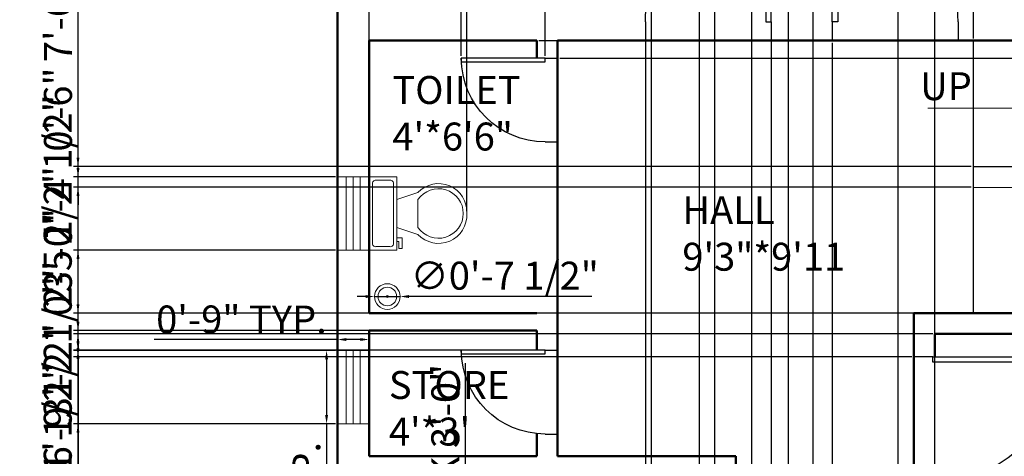
# Model space of a CAD drawing. Units: inches. Extents: x 2528 to 2954, y 1660 to 2209.
# Tile 2 of 4: x 2528 to 2810, y 1832 to 1957. Entities that reach past the tile are written whole.
import ezdxf

# ---------------------------------------------------------------- set-up
doc = ezdxf.new("R2010")
doc.units = ezdxf.units.IN
for name, color, linetype, lineweight in [('A-ANNO-DIMS', 5, 'Continuous', 18), ('A-ANNO-SYMB', 5, 'Continuous', 18), ('A-AREA-IDEN', 5, 'Continuous', 25), ('A-FLOR-FIXT', 6, 'Continuous', 18), ('DOOR', 3, 'Continuous', 25), ('STEPS', 30, 'Continuous', 25), ('TEXT', 5, 'Continuous', 25), ('WALL', 1, 'Continuous', 50), ('WINDOW', 4, 'Continuous', 18)]:
    doc.layers.add(name, color=color, linetype=linetype, lineweight=lineweight)
doc.styles.get("Standard").update_dxf_attribs({"font": 'arial.ttf'})
doc.dimstyles.new('ISO-25', dxfattribs={"dimtxt": 8, "dimasz": 2.5, "dimexe": 1.25, "dimexo": 0.625, "dimtad": 1, "dimlunit": 3, "dimtxsty": 'Standard', "dimcen": 2.5, "dimadec": 0, "dimazin": 0, "dimtfac": 1, "dimtmove": 0, "dimatfit": 3, "dimfxl": 1, "dimarcsym": 0})

# ---------------------------------------------------------------- blocks, each defined once
blk = doc.blocks.new('*U2')
for p, q in [((0, 0), (0, -6)), ((40, 0), (40, -6))]:
    blk.add_line(p, q)
blk.add_lwpolyline([(0, 0), (0, 40), (1.75, 40), (1.75, 0)], close=True)
blk.add_arc((0, 0), 40, 0, 90)
blk = doc.blocks.new('*U4')
for p, q in [((9.5, -6), (9.5, -2)), ((-8, -8.5), (-8, -8)), ((-7, -8), (-7, -9.5)), ((-4, -8), (-6, -14)), ((4, -8), (6, -14)), ((-10, -8.5), (-8, -8.5)), ((-10, -9.5), (-10, -8.5)), ((-7, -9.5), (-10, -9.5)), ((4, -14), (-4, -14))]:
    blk.add_line(p, q)
blk.add_lwpolyline([(10.5, -8), (10.5, 0), (-10.5, 0), (-10.5, -8)], close=True)
for points in [[(-9.5, -2), (-9.5, -6)], [(8.5, -1), (-8.5, -1)], [(-8.5, -7), (8.5, -7)]]:
    blk.add_lwpolyline(points)
for centre, radius, start, end in [((-8.625, -1.875), 0.8839, 81.8699, 188.1301), ((8.625, -1.875), 0.8839, 351.8699, 98.1301), ((-8.625, -6.125), 0.8839, 171.869898, 278.1301), ((8.625, -6.125), 0.8839, 261.8699, 8.1301), ((-0.4772, -19.9188), 8.0953, 133.01722, 273.38), ((0.0374, -19.8731), 7.127, 124.50543, 269.7), ((-0.0373, -19.8731), 7.127, 270.3, 55.4946), ((0.4773, -19.9188), 8.0953, 266.62, 46.9828)]:
    blk.add_arc(centre, radius, start, end)
blk = doc.blocks.new('WIN-21IN')
for p, q in [((9, 21), (0, 21)), ((2.5, 21), (2.5, 0)), ((4.5, 21), (4.5, 0)), ((6.5, 21), (6.5, 0)), ((9, 0), (0, 0))]:
    blk.add_line(p, q)
blk = doc.blocks.new('*D19')
at = {"layer": 'A-ANNO-DIMS', "color": 0, "lineweight": -2, "transparency": 16777216}
for p, q in [((2618.29, 1862.65), (2614.52, 1862.65)), ((2615.77, 1860.15), (2615.77, 1844.15)), ((2618.29, 1841.65), (2614.52, 1841.65)), ((2615.77, 1841.65), (2615.77, 1736.66))]:
    blk.add_line(p, q, dxfattribs=at)
at = {"layer": 'A-ANNO-DIMS', "color": 0, "transparency": 16777216}
for points in [[(2615.35, 1860.15), (2616.18, 1860.15), (2615.77, 1862.65)], [(2615.35, 1844.15), (2616.18, 1844.15), (2615.77, 1841.65)]]:
    blk.add_solid(points, dxfattribs=at)
at = {"layer": 'Defpoints', "color": 0, "transparency": 16777216}
for p in [(2618.92, 1862.65), (2615.77, 1841.65), (2618.92, 1841.65)]:
    blk.add_point(p, dxfattribs=at)
at = {"layer": 'A-ANNO-DIMS', "color": 0, "transparency": 16777216, "insert": (2611, 1787.9), "char_height": 8, "attachment_point": 5, "rotation": 90}
blk.add_mtext('WINDOW 1\'-9" TYP.', dxfattribs=at)
blk = doc.blocks.new('*D20')
at = {"layer": 'A-ANNO-DIMS', "color": 0, "lineweight": -2, "transparency": 16777216}
for p, q in [((2618.92, 1863.27), (2618.92, 1867.05)), ((2627.92, 1863.27), (2627.92, 1867.05)), ((2618.92, 1865.8), (2566.4, 1865.8)), ((2625.42, 1865.8), (2621.42, 1865.8))]:
    blk.add_line(p, q, dxfattribs=at)
at = {"layer": 'A-ANNO-DIMS', "color": 0, "transparency": 16777216}
for points in [[(2621.42, 1866.21), (2621.42, 1865.38), (2618.92, 1865.8)], [(2625.42, 1866.21), (2625.42, 1865.38), (2627.92, 1865.8)]]:
    blk.add_solid(points, dxfattribs=at)
at = {"layer": 'Defpoints', "color": 0, "transparency": 16777216}
for p in [(2618.92, 1865.8), (2618.92, 1862.65), (2627.92, 1862.65)]:
    blk.add_point(p, dxfattribs=at)
at = {"layer": 'A-ANNO-DIMS', "color": 0, "transparency": 16777216, "insert": (2591.41, 1870.5), "char_height": 8, "attachment_point": 5}
blk.add_mtext('0\'-9" TYP.', dxfattribs=at)
blk = doc.blocks.new('*D23')
at = {"layer": 'A-ANNO-DIMS', "color": 0, "lineweight": -2, "transparency": 16777216}
for p, q in [((2655.56, 1804.89), (2655.56, 1859.06)), ((2650.79, 1804.89), (2656.81, 1804.89)), ((2655.56, 1771.39), (2655.56, 1802.39)), ((2650.79, 1768.89), (2656.81, 1768.89))]:
    blk.add_line(p, q, dxfattribs=at)
at = {"layer": 'A-ANNO-DIMS', "color": 0, "transparency": 16777216}
for points in [[(2655.15, 1802.39), (2655.98, 1802.39), (2655.56, 1804.89)], [(2655.15, 1771.39), (2655.98, 1771.39), (2655.56, 1768.89)]]:
    blk.add_solid(points, dxfattribs=at)
at = {"layer": 'Defpoints', "color": 0, "transparency": 16777216}
for p in [(2650.16, 1804.89), (2655.56, 1804.89), (2650.16, 1768.89)]:
    blk.add_point(p, dxfattribs=at)
at = {"layer": 'A-ANNO-DIMS', "color": 0, "transparency": 16777216, "insert": (2650.8, 1833.22), "char_height": 8, "attachment_point": 5, "rotation": 90}
blk.add_mtext('SINK 3\'-0"', dxfattribs=at)
blk = doc.blocks.new('*D28')
at = {"layer": 'A-ANNO-DIMS', "color": 0, "lineweight": -2, "transparency": 16777216}
for p, q in [((2544.62, 1841.65), (2544.62, 1885.3)), ((2618.29, 1841.65), (2543.37, 1841.65)), ((2544.62, 1805.43), (2544.62, 1839.14)), ((2618.29, 1802.93), (2543.37, 1802.93))]:
    blk.add_line(p, q, dxfattribs=at)
at = {"layer": 'A-ANNO-DIMS', "color": 0, "transparency": 16777216}
for points in [[(2544.2, 1839.14), (2545.03, 1839.14), (2544.62, 1841.65)], [(2544.2, 1805.43), (2545.03, 1805.43), (2544.62, 1802.93)]]:
    blk.add_solid(points, dxfattribs=at)
at = {"layer": 'Defpoints', "color": 0, "transparency": 16777216}
for p in [(2544.62, 1841.65), (2618.92, 1841.65), (2618.92, 1802.93)]:
    blk.add_point(p, dxfattribs=at)
at = {"layer": 'A-ANNO-DIMS', "color": 0, "transparency": 16777216, "insert": (2539.85, 1864.72), "char_height": 8, "attachment_point": 5, "rotation": 90}
blk.add_mtext('3\'-2 1/2"', dxfattribs=at)
blk = doc.blocks.new('*D29')
at = {"layer": 'A-ANNO-DIMS', "color": 0, "lineweight": -2, "transparency": 16777216}
for p, q in [((2544.62, 1891.39), (2544.62, 1935.18)), ((2618.29, 1891.39), (2543.37, 1891.39)), ((2544.62, 1865.15), (2544.62, 1888.89)), ((2618.29, 1862.64), (2543.37, 1862.64))]:
    blk.add_line(p, q, dxfattribs=at)
at = {"layer": 'A-ANNO-DIMS', "color": 0, "transparency": 16777216}
for points in [[(2544.2, 1888.89), (2545.03, 1888.89), (2544.62, 1891.39)], [(2544.2, 1865.15), (2545.03, 1865.15), (2544.62, 1862.64)]]:
    blk.add_solid(points, dxfattribs=at)
at = {"layer": 'Defpoints', "color": 0, "transparency": 16777216}
for p in [(2544.62, 1891.39), (2618.92, 1891.39), (2618.92, 1862.64)]:
    blk.add_point(p, dxfattribs=at)
at = {"layer": 'A-ANNO-DIMS', "color": 0, "transparency": 16777216, "insert": (2539.85, 1914.54), "char_height": 8, "attachment_point": 5, "rotation": 90}
blk.add_mtext('2\'-4 1/2"', dxfattribs=at)
blk = doc.blocks.new('*D30')
at = {"layer": 'A-ANNO-DIMS', "color": 0, "lineweight": -2, "transparency": 16777216}
for p, q in [((2618.29, 2002.2), (2543.37, 2002.2)), ((2544.62, 1914.89), (2544.62, 1999.7)), ((2618.29, 1912.39), (2543.37, 1912.39))]:
    blk.add_line(p, q, dxfattribs=at)
at = {"layer": 'A-ANNO-DIMS', "color": 0, "transparency": 16777216}
for points in [[(2544.2, 1999.7), (2545.03, 1999.7), (2544.62, 2002.2)], [(2544.2, 1914.89), (2545.03, 1914.89), (2544.62, 1912.39)]]:
    blk.add_solid(points, dxfattribs=at)
at = {"layer": 'Defpoints', "color": 0, "transparency": 16777216}
for p in [(2544.62, 2002.2), (2618.92, 2002.2), (2618.92, 1912.39)]:
    blk.add_point(p, dxfattribs=at)
at = {"layer": 'A-ANNO-DIMS', "color": 0, "transparency": 16777216, "insert": (2539.91, 1957.29), "char_height": 8, "attachment_point": 5, "rotation": 90}
blk.add_mtext('7\'-6"', dxfattribs=at)
blk = doc.blocks.new('*D34')
at = {"layer": 'A-ANNO-DIMS', "color": 0, "lineweight": -2, "transparency": 16777216}
for p, q in [((2618.92, 1715.01), (2618.92, 2122.94)), ((2726.92, 1703.01), (2726.92, 2122.94)), ((2621.42, 2121.69), (2724.42, 2121.69))]:
    blk.add_line(p, q, dxfattribs=at)
at = {"layer": 'A-ANNO-DIMS', "color": 0, "transparency": 16777216}
for points in [[(2621.42, 2122.11), (2621.42, 2121.27), (2618.92, 2121.69)], [(2724.42, 2122.11), (2724.42, 2121.27), (2726.92, 2121.69)]]:
    blk.add_solid(points, dxfattribs=at)
at = {"layer": 'Defpoints', "color": 0, "transparency": 16777216}
for p in [(2726.92, 2121.69), (2618.92, 1714.39), (2726.92, 1702.39)]:
    blk.add_point(p, dxfattribs=at)
at = {"layer": 'A-ANNO-DIMS', "color": 0, "transparency": 16777216, "insert": (2672.92, 2126.4), "char_height": 8, "attachment_point": 5}
blk.add_mtext('9\'-0"', dxfattribs=at)
blk = doc.blocks.new('*D35')
at = {"layer": 'A-ANNO-DIMS', "color": 0, "lineweight": -2, "transparency": 16777216}
for p, q in [((2726.92, 1691.01), (2726.92, 2122.94)), ((2789.92, 1691.01), (2789.92, 2122.94)), ((2729.42, 2121.69), (2787.42, 2121.69))]:
    blk.add_line(p, q, dxfattribs=at)
at = {"layer": 'A-ANNO-DIMS', "color": 0, "transparency": 16777216}
for points in [[(2729.42, 2122.11), (2729.42, 2121.27), (2726.92, 2121.69)], [(2787.42, 2122.11), (2787.42, 2121.27), (2789.92, 2121.69)]]:
    blk.add_solid(points, dxfattribs=at)
at = {"layer": 'Defpoints', "color": 0, "transparency": 16777216}
for p in [(2789.92, 2121.69), (2726.92, 1690.39), (2789.92, 1690.39)]:
    blk.add_point(p, dxfattribs=at)
at = {"layer": 'A-ANNO-DIMS', "color": 0, "transparency": 16777216, "insert": (2758.42, 2126.4), "char_height": 8, "attachment_point": 5}
blk.add_mtext('5\'-3"', dxfattribs=at)
blk = doc.blocks.new('*D37')
at = {"layer": 'A-ANNO-DIMS', "color": 0, "lineweight": -2, "transparency": 16777216}
for p, q in [((2737.46, 1724.01), (2737.46, 2122.94)), ((2779.37, 1724.01), (2779.37, 2122.94)), ((2739.96, 2121.69), (2776.87, 2121.69))]:
    blk.add_line(p, q, dxfattribs=at)
at = {"layer": 'A-ANNO-DIMS', "color": 0, "transparency": 16777216}
for points in [[(2739.96, 2122.11), (2739.96, 2121.27), (2737.46, 2121.69)], [(2776.87, 2122.11), (2776.87, 2121.27), (2779.37, 2121.69)]]:
    blk.add_solid(points, dxfattribs=at)
at = {"layer": 'Defpoints', "color": 0, "transparency": 16777216}
for p in [(2779.37, 2121.69), (2737.46, 1723.39), (2779.37, 1723.39)]:
    blk.add_point(p, dxfattribs=at)
at = {"layer": 'A-ANNO-DIMS', "color": 0, "transparency": 16777216, "insert": (2758.42, 2126.4), "char_height": 8, "attachment_point": 5}
blk.add_mtext('3\'-6"', dxfattribs=at)
blk = doc.blocks.new('*D38')
at = {"layer": 'A-ANNO-DIMS', "color": 0, "lineweight": -2, "transparency": 16777216}
for p, q in [((2707.05, 1956.76), (2707.05, 1665.84)), ((2743.05, 1956.76), (2743.05, 1665.84)), ((2709.55, 1667.09), (2740.55, 1667.09))]:
    blk.add_line(p, q, dxfattribs=at)
at = {"layer": 'A-ANNO-DIMS', "color": 0, "transparency": 16777216}
for points in [[(2709.55, 1667.51), (2709.55, 1666.67), (2707.05, 1667.09)], [(2740.55, 1667.51), (2740.55, 1666.67), (2743.05, 1667.09)]]:
    blk.add_solid(points, dxfattribs=at)
at = {"layer": 'Defpoints', "color": 0, "transparency": 16777216}
for p in [(2707.05, 1957.39), (2743.05, 1957.39), (2743.05, 1667.09)]:
    blk.add_point(p, dxfattribs=at)
at = {"layer": 'A-ANNO-DIMS', "color": 0, "transparency": 16777216, "insert": (2725.05, 1671.8), "char_height": 8, "attachment_point": 5}
blk.add_mtext('3\'-0"', dxfattribs=at)
blk = doc.blocks.new('*D39')
at = {"layer": 'A-ANNO-DIMS', "color": 0, "lineweight": -2, "transparency": 16777216}
for p, q in [((2654.34, 1947.01), (2654.34, 2122.94)), ((2678.32, 1947.01), (2678.32, 2122.94)), ((2656.84, 2121.69), (2675.82, 2121.69))]:
    blk.add_line(p, q, dxfattribs=at)
at = {"layer": 'A-ANNO-DIMS', "color": 0, "transparency": 16777216}
for points in [[(2656.84, 2122.11), (2656.84, 2121.27), (2654.34, 2121.69)], [(2675.82, 2122.11), (2675.82, 2121.27), (2678.32, 2121.69)]]:
    blk.add_solid(points, dxfattribs=at)
at = {"layer": 'Defpoints', "color": 0, "transparency": 16777216}
for p in [(2678.32, 2121.69), (2654.34, 1946.38), (2678.32, 1946.38)]:
    blk.add_point(p, dxfattribs=at)
at = {"layer": 'A-ANNO-DIMS', "color": 0, "transparency": 16777216, "insert": (2666.33, 2126.4), "char_height": 8, "attachment_point": 5}
blk.add_mtext('2\'-0"', dxfattribs=at)
blk = doc.blocks.new('*D41')
at = {"layer": 'A-ANNO-DIMS', "color": 0, "lineweight": -2, "transparency": 16777216}
for p, q in [((2800.92, 1952.01), (2800.92, 2122.94)), ((2877.42, 1952.01), (2877.42, 2122.94)), ((2803.42, 2121.69), (2874.92, 2121.69))]:
    blk.add_line(p, q, dxfattribs=at)
at = {"layer": 'A-ANNO-DIMS', "color": 0, "transparency": 16777216}
for points in [[(2803.42, 2122.11), (2803.42, 2121.27), (2800.92, 2121.69)], [(2874.92, 2122.11), (2874.92, 2121.27), (2877.42, 2121.69)]]:
    blk.add_solid(points, dxfattribs=at)
at = {"layer": 'Defpoints', "color": 0, "transparency": 16777216}
for p in [(2877.42, 2121.69), (2800.92, 1951.39), (2877.42, 1951.39)]:
    blk.add_point(p, dxfattribs=at)
at = {"layer": 'A-ANNO-DIMS', "color": 0, "transparency": 16777216, "insert": (2839.17, 2126.45), "char_height": 8, "attachment_point": 5}
blk.add_mtext('6\'-4 1/2"', dxfattribs=at)
blk = doc.blocks.new('*D42')
at = {"layer": 'A-ANNO-DIMS', "color": 0, "lineweight": -2, "transparency": 16777216}
for p, q in [((2800.28, 1909.39), (2543.37, 1909.39)), ((2544.62, 1875.89), (2544.62, 1906.89)), ((2800.29, 1873.39), (2543.37, 1873.39))]:
    blk.add_line(p, q, dxfattribs=at)
at = {"layer": 'A-ANNO-DIMS', "color": 0, "transparency": 16777216}
for points in [[(2544.2, 1906.89), (2545.03, 1906.89), (2544.62, 1909.39)], [(2544.2, 1875.89), (2545.03, 1875.89), (2544.62, 1873.39)]]:
    blk.add_solid(points, dxfattribs=at)
at = {"layer": 'Defpoints', "color": 0, "transparency": 16777216}
for p in [(2544.62, 1909.39), (2800.9, 1909.39), (2800.92, 1873.39)]:
    blk.add_point(p, dxfattribs=at)
at = {"layer": 'A-ANNO-DIMS', "color": 0, "transparency": 16777216, "insert": (2539.9, 1891.39), "char_height": 8, "attachment_point": 5, "rotation": 90}
blk.add_mtext('3\'-0"', dxfattribs=at)
blk = doc.blocks.new('*D45')
at = {"layer": 'A-ANNO-DIMS', "color": 0, "lineweight": -2, "transparency": 16777216}
for p, q in [((2708.76, 1744.99), (2708.76, 2122.94)), ((2726.92, 1748.01), (2726.92, 2122.94)), ((2711.26, 2121.69), (2724.42, 2121.69)), ((2726.92, 2121.69), (2751.18, 2121.69))]:
    blk.add_line(p, q, dxfattribs=at)
at = {"layer": 'A-ANNO-DIMS', "color": 0, "transparency": 16777216}
for points in [[(2711.26, 2122.11), (2711.26, 2121.27), (2708.76, 2121.69)], [(2724.42, 2122.11), (2724.42, 2121.27), (2726.92, 2121.69)]]:
    blk.add_solid(points, dxfattribs=at)
at = {"layer": 'Defpoints', "color": 0, "transparency": 16777216}
for p in [(2726.92, 2121.69), (2726.92, 1747.39), (2708.76, 1744.37)]:
    blk.add_point(p, dxfattribs=at)
at = {"layer": 'A-ANNO-DIMS', "color": 0, "transparency": 16777216, "insert": (2740.3, 2126.4), "char_height": 8, "attachment_point": 5}
blk.add_mtext('1\'-6"', dxfattribs=at)
blk = doc.blocks.new('*D46')
at = {"layer": 'A-ANNO-DIMS', "color": 0, "lineweight": -2, "transparency": 16777216}
for p, q in [((2544.62, 1826.39), (2544.62, 1869.29)), ((2627.29, 1826.39), (2543.37, 1826.39)), ((2544.62, 1807.39), (2544.62, 1823.89)), ((2630.04, 1804.89), (2543.37, 1804.89))]:
    blk.add_line(p, q, dxfattribs=at)
at = {"layer": 'A-ANNO-DIMS', "color": 0, "transparency": 16777216}
for points in [[(2544.2, 1823.89), (2545.03, 1823.89), (2544.62, 1826.39)], [(2544.2, 1807.39), (2545.03, 1807.39), (2544.62, 1804.89)]]:
    blk.add_solid(points, dxfattribs=at)
at = {"layer": 'Defpoints', "color": 0, "transparency": 16777216}
for p in [(2544.62, 1826.39), (2627.92, 1826.39), (2630.66, 1804.89)]:
    blk.add_point(p, dxfattribs=at)
at = {"layer": 'A-ANNO-DIMS', "color": 0, "transparency": 16777216, "insert": (2539.85, 1849.09), "char_height": 8, "attachment_point": 5, "rotation": 90}
blk.add_mtext('1\'-9 1/2"', dxfattribs=at)
blk = doc.blocks.new('*D47')
at = {"layer": 'A-ANNO-DIMS', "color": 0, "lineweight": -2, "transparency": 16777216}
for p, q in [((2627.92, 1913.01), (2627.92, 2122.94)), ((2655.91, 1902.51), (2655.91, 2122.94)), ((2653.41, 2121.69), (2630.42, 2121.69))]:
    blk.add_line(p, q, dxfattribs=at)
at = {"layer": 'A-ANNO-DIMS', "color": 0, "transparency": 16777216}
for points in [[(2630.42, 2122.11), (2630.42, 2121.27), (2627.92, 2121.69)], [(2653.41, 2122.11), (2653.41, 2121.27), (2655.91, 2121.69)]]:
    blk.add_solid(points, dxfattribs=at)
at = {"layer": 'Defpoints', "color": 0, "transparency": 16777216}
for p in [(2627.92, 2121.69), (2627.92, 1912.39), (2655.91, 1901.89)]:
    blk.add_point(p, dxfattribs=at)
at = {"layer": 'A-ANNO-DIMS', "color": 0, "transparency": 16777216, "insert": (2641.91, 2126.33), "char_height": 8, "attachment_point": 5}
blk.add_mtext('2\'-4"', dxfattribs=at)
blk = doc.blocks.new('*D48')
at = {"layer": 'A-ANNO-DIMS', "color": 0, "lineweight": -2, "transparency": 16777216}
for p, q in [((2747.92, 2088.76), (2747.92, 1665.84)), ((2754.92, 2088.76), (2754.92, 1665.84)), ((2750.42, 1667.09), (2752.42, 1667.09)), ((2754.92, 1667.09), (2779.93, 1667.09))]:
    blk.add_line(p, q, dxfattribs=at)
at = {"layer": 'A-ANNO-DIMS', "color": 0, "transparency": 16777216}
for points in [[(2750.42, 1667.51), (2750.42, 1666.67), (2747.92, 1667.09)], [(2752.42, 1667.51), (2752.42, 1666.67), (2754.92, 1667.09)]]:
    blk.add_solid(points, dxfattribs=at)
at = {"layer": 'Defpoints', "color": 0, "transparency": 16777216}
for p in [(2747.92, 2089.39), (2754.92, 2089.39), (2754.92, 1667.09)]:
    blk.add_point(p, dxfattribs=at)
at = {"layer": 'A-ANNO-DIMS', "color": 0, "transparency": 16777216, "insert": (2768.67, 1671.8), "char_height": 8, "attachment_point": 5}
blk.add_mtext('0\'-7"', dxfattribs=at)
blk = doc.blocks.new('*D49')
at = {"layer": 'A-ANNO-DIMS', "color": 0, "lineweight": -2, "transparency": 16777216}
for p, q in [((2747.92, 1956.76), (2747.92, 1665.84)), ((2743.05, 1950.76), (2743.05, 1665.84)), ((2740.55, 1667.09), (2738.05, 1667.09)), ((2743.05, 1667.09), (2747.92, 1667.09)), ((2750.42, 1667.09), (2775.43, 1667.09))]:
    blk.add_line(p, q, dxfattribs=at)
at = {"layer": 'A-ANNO-DIMS', "color": 0, "transparency": 16777216}
for points in [[(2740.55, 1667.51), (2740.55, 1666.67), (2743.05, 1667.09)], [(2750.42, 1667.51), (2750.42, 1666.67), (2747.92, 1667.09)]]:
    blk.add_solid(points, dxfattribs=at)
at = {"layer": 'Defpoints', "color": 0, "transparency": 16777216}
for p in [(2747.92, 1957.39), (2743.05, 1951.39), (2747.92, 1667.09)]:
    blk.add_point(p, dxfattribs=at)
at = {"layer": 'A-ANNO-DIMS', "color": 0, "transparency": 16777216, "insert": (2764.17, 1671.8), "char_height": 8, "attachment_point": 5}
blk.add_mtext('0\'-5"', dxfattribs=at)
blk = doc.blocks.new('*D50')
at = {"layer": 'A-ANNO-DIMS', "color": 0, "lineweight": -2, "transparency": 16777216}
for p, q in [((2754.92, 1956.76), (2754.92, 1665.84)), ((2760.54, 1950.76), (2760.54, 1665.84)), ((2752.42, 1667.09), (2749.92, 1667.09)), ((2754.92, 1667.09), (2760.54, 1667.09)), ((2763.04, 1667.09), (2806.7, 1667.09))]:
    blk.add_line(p, q, dxfattribs=at)
at = {"layer": 'A-ANNO-DIMS', "color": 0, "transparency": 16777216}
for points in [[(2752.42, 1667.51), (2752.42, 1666.67), (2754.92, 1667.09)], [(2763.04, 1667.51), (2763.04, 1666.67), (2760.54, 1667.09)]]:
    blk.add_solid(points, dxfattribs=at)
at = {"layer": 'Defpoints', "color": 0, "transparency": 16777216}
for p in [(2754.92, 1957.39), (2760.54, 1951.39), (2760.54, 1667.09)]:
    blk.add_point(p, dxfattribs=at)
at = {"layer": 'A-ANNO-DIMS', "color": 0, "transparency": 16777216, "insert": (2786.12, 1671.85), "char_height": 8, "attachment_point": 5}
blk.add_mtext('0\'-5 1/2"', dxfattribs=at)
blk = doc.blocks.new('*D51')
at = {"layer": 'A-ANNO-DIMS', "color": 0, "lineweight": -2, "transparency": 16777216}
for p, q in [((2789.29, 1867.39), (2543.37, 1867.39)), ((2544.62, 1864.89), (2544.62, 1863.37)), ((2783.29, 1860.87), (2543.37, 1860.87)), ((2544.62, 1860.87), (2544.62, 1817.21))]:
    blk.add_line(p, q, dxfattribs=at)
at = {"layer": 'A-ANNO-DIMS', "color": 0, "transparency": 16777216}
for points in [[(2544.2, 1864.89), (2545.03, 1864.89), (2544.62, 1867.39)], [(2544.2, 1863.37), (2545.03, 1863.37), (2544.62, 1860.87)]]:
    blk.add_solid(points, dxfattribs=at)
at = {"layer": 'Defpoints', "color": 0, "transparency": 16777216}
for p in [(2789.92, 1867.39), (2544.62, 1860.87), (2783.92, 1860.87)]:
    blk.add_point(p, dxfattribs=at)
at = {"layer": 'A-ANNO-DIMS', "color": 0, "transparency": 16777216, "insert": (2539.85, 1837.79), "char_height": 8, "attachment_point": 5, "rotation": 90}
blk.add_mtext('0\'-6 1/2"', dxfattribs=at)
blk = doc.blocks.new('*D52')
at = {"layer": 'A-ANNO-DIMS', "color": 0, "lineweight": -2, "transparency": 16777216}
for p, q in [((2942.22, 1953.89), (2942.22, 1978.91)), ((2676.54, 1951.39), (2943.47, 1951.39)), ((2942.22, 1946.38), (2942.22, 1951.39)), ((2682.54, 1946.38), (2943.47, 1946.38)), ((2942.22, 1943.88), (2942.22, 1941.38))]:
    blk.add_line(p, q, dxfattribs=at)
at = {"layer": 'A-ANNO-DIMS', "color": 0, "transparency": 16777216}
for points in [[(2941.8, 1953.89), (2942.63, 1953.89), (2942.22, 1951.39)], [(2941.8, 1943.88), (2942.63, 1943.88), (2942.22, 1946.38)]]:
    blk.add_solid(points, dxfattribs=at)
at = {"layer": 'Defpoints', "color": 0, "transparency": 16777216}
for p in [(2675.92, 1951.39), (2942.22, 1951.39), (2681.92, 1946.38)]:
    blk.add_point(p, dxfattribs=at)
at = {"layer": 'A-ANNO-DIMS', "color": 0, "transparency": 16777216, "insert": (2937.51, 1967.65), "char_height": 8, "attachment_point": 5, "rotation": 90}
blk.add_mtext('0\'-5"', dxfattribs=at)
blk = doc.blocks.new('*D53')
at = {"layer": 'A-ANNO-DIMS', "color": 0, "lineweight": -2, "transparency": 16777216}
for p, q in [((2544.62, 1870.89), (2544.62, 1914.55)), ((2675.29, 1868.39), (2543.37, 1868.39)), ((2544.62, 1862.71), (2544.62, 1868.39)), ((2675.29, 1862.71), (2543.37, 1862.71)), ((2544.62, 1860.21), (2544.62, 1857.71))]:
    blk.add_line(p, q, dxfattribs=at)
at = {"layer": 'A-ANNO-DIMS', "color": 0, "transparency": 16777216}
for points in [[(2544.2, 1870.89), (2545.03, 1870.89), (2544.62, 1868.39)], [(2544.2, 1860.21), (2545.03, 1860.21), (2544.62, 1862.71)]]:
    blk.add_solid(points, dxfattribs=at)
at = {"layer": 'Defpoints', "color": 0, "transparency": 16777216}
for p in [(2544.62, 1868.39), (2675.92, 1868.39), (2675.92, 1862.71)]:
    blk.add_point(p, dxfattribs=at)
at = {"layer": 'A-ANNO-DIMS', "color": 0, "transparency": 16777216, "insert": (2539.85, 1893.97), "char_height": 8, "attachment_point": 5, "rotation": 90}
blk.add_mtext('0\'-5 1/2"', dxfattribs=at)
blk = doc.blocks.new('*D54')
at = {"layer": 'A-ANNO-DIMS', "color": 0, "lineweight": -2, "transparency": 16777216}
for p, q in [((2722.51, 1827.01), (2722.51, 2122.94)), ((2726.92, 1827.01), (2726.92, 2122.94)), ((2720.01, 2121.69), (2717.51, 2121.69)), ((2722.51, 2121.69), (2726.92, 2121.69)), ((2729.42, 2121.69), (2773.07, 2121.69))]:
    blk.add_line(p, q, dxfattribs=at)
at = {"layer": 'A-ANNO-DIMS', "color": 0, "transparency": 16777216}
for points in [[(2720.01, 2122.11), (2720.01, 2121.27), (2722.51, 2121.69)], [(2729.42, 2122.11), (2729.42, 2121.27), (2726.92, 2121.69)]]:
    blk.add_solid(points, dxfattribs=at)
at = {"layer": 'Defpoints', "color": 0, "transparency": 16777216}
for p in [(2726.92, 2121.69), (2722.51, 1826.39), (2726.92, 1826.39)]:
    blk.add_point(p, dxfattribs=at)
at = {"layer": 'A-ANNO-DIMS', "color": 0, "transparency": 16777216, "insert": (2752.49, 2126.45), "char_height": 8, "attachment_point": 5}
blk.add_mtext('0\'-4 1/2"', dxfattribs=at)
blk = doc.blocks.new('*D56')
at = {"layer": 'A-ANNO-DIMS', "color": 0, "lineweight": -2, "transparency": 16777216}
for p, q in [((2544.62, 1917.89), (2544.62, 1942.91)), ((2800.3, 1915.39), (2543.37, 1915.39)), ((2544.62, 1909.39), (2544.62, 1915.39)), ((2800.28, 1909.39), (2543.37, 1909.39)), ((2544.62, 1906.89), (2544.62, 1904.39))]:
    blk.add_line(p, q, dxfattribs=at)
at = {"layer": 'A-ANNO-DIMS', "color": 0, "transparency": 16777216}
for points in [[(2544.2, 1917.89), (2545.03, 1917.89), (2544.62, 1915.39)], [(2544.2, 1906.89), (2545.03, 1906.89), (2544.62, 1909.39)]]:
    blk.add_solid(points, dxfattribs=at)
at = {"layer": 'Defpoints', "color": 0, "transparency": 16777216}
for p in [(2544.62, 1915.39), (2800.93, 1915.39), (2800.9, 1909.39)]:
    blk.add_point(p, dxfattribs=at)
at = {"layer": 'A-ANNO-DIMS', "color": 0, "transparency": 16777216, "insert": (2539.91, 1931.65), "char_height": 8, "attachment_point": 5, "rotation": 90}
blk.add_mtext('0\'-6"', dxfattribs=at)
blk = doc.blocks.new('*D57')
at = {"layer": 'A-ANNO-DIMS', "color": 0, "lineweight": -2, "transparency": 16777216}
for p, q in [((2627, 1878.11), (2624.5, 1878.11)), ((2629.5, 1878.11), (2636.83, 1878.11)), ((2691.69, 1878.11), (2639.33, 1878.11))]:
    blk.add_line(p, q, dxfattribs=at)
at = {"layer": 'A-ANNO-DIMS', "color": 0, "transparency": 16777216}
for points in [[(2627, 1878.52), (2627, 1877.69), (2629.5, 1878.11)], [(2639.33, 1878.52), (2639.33, 1877.69), (2636.83, 1878.11)]]:
    blk.add_solid(points, dxfattribs=at)
at = {"layer": 'Defpoints', "color": 0, "transparency": 16777216}
for p in [(2629.5, 1878.11), (2636.83, 1878.11)]:
    blk.add_point(p, dxfattribs=at)
at = {"layer": 'A-ANNO-DIMS', "color": 0, "transparency": 16777216, "insert": (2666.76, 1883.04), "char_height": 8, "attachment_point": 5, "rotation": 0.0045}
blk.add_mtext('∅0\'-7 1/2"', dxfattribs=at)

msp = doc.modelspace()

# ---------------------------------------------------------------- linework, layer by layer
at = {"layer": 'A-ANNO-SYMB'}
msp.add_line((2787.908, 1932.092), (2877.423, 1932.092), dxfattribs=at)
at = {"layer": 'A-FLOR-FIXT'}
for radius in [3.668, 2.668, 0.311, 0.111]:
    msp.add_circle((2633.164, 1878.108), radius, dxfattribs=at)
at = {"layer": 'STEPS'}
for p, q in [((2800.915, 1873.389), (2800.915, 1951.389)), ((2800.929, 1915.389), (2877.423, 1915.038)), ((2800.901, 1909.389), (2877.423, 1909.038))]:
    msp.add_line(p, q, dxfattribs=at)
at = {"layer": 'WALL'}
for p, q in [((2627.915, 1951.389), (2675.915, 1951.389)), ((2627.915, 1873.389), (2627.915, 1951.389)), ((2675.915, 1946.385), (2675.915, 1951.389)), ((2681.915, 1832.389), (2681.915, 1951.389)), ((2681.915, 1951.389), (2909.915, 1951.389)), ((2627.915, 1873.389), (2675.915, 1873.389)), ((2783.915, 1873.389), (2783.915, 1723.389)), ((2783.915, 1873.389), (2909.915, 1873.389)), ((2627.915, 1832.389), (2627.915, 1868.389)), ((2675.915, 1868.389), (2627.915, 1868.389)), ((2675.915, 1862.714), (2675.915, 1868.389)), ((2909.915, 1867.389), (2789.915, 1867.389)), ((2789.915, 1867.389), (2789.915, 1860.866)), ((2675.915, 1832.389), (2675.915, 1838.855)), ((2675.915, 1832.389), (2627.915, 1832.389)), ((2732.915, 1832.389), (2681.915, 1832.389)), ((2732.915, 1723.389), (2732.915, 1832.389))]:
    msp.add_line(p, q, dxfattribs=at)
msp.add_lwpolyline([(2618.915, 2098.389), (2918.915, 2098.389), (2918.915, 1714.389), (2618.915, 1714.389)], close=True, dxfattribs=at)

# ---------------------------------------------------------------- block references
at = {"layer": 'A-FLOR-FIXT', "rotation": 90.00000000000063}
msp.add_blockref('*U4', (2627.915, 1901.889), dxfattribs=at)
at = {"layer": 'DOOR', "yscale": 0.9, "zscale": 0.9}
for p, xscale in [((2743.048, 1956.789), -0.9), ((2760.539, 1956.789), 0.9)]:
    msp.add_blockref('*U2', p, dxfattribs=dict(at, xscale=xscale))
at = {"layer": 'DOOR'}
for p, xscale, yscale, zscale, rotation in [((2678.318, 1946.385), -0.5994989179374447, 0.5994989179374447, 0.5994989179374447, 90), ((2678.318, 1862.714), -0.5994989179374447, 0.5994989179374447, 0.5994989179374447, 90), ((2789.315, 1860.866), 0.9, 0.9, 0.9, 270)]:
    msp.add_blockref('*U2', p, dxfattribs=dict(at, xscale=xscale, yscale=yscale, zscale=zscale, rotation=rotation))
at = {"layer": 'WINDOW'}
msp.add_blockref('WIN-21IN', (2618.915, 1891.389), dxfattribs=at)
at = {"layer": 'WINDOW', "rotation": 180}
msp.add_blockref('WIN-21IN', (2627.915, 1862.645), dxfattribs=at)

# ---------------------------------------------------------------- texts
at = {"layer": 'A-AREA-IDEN', "char_height": 8, "attachment_point": 1}
for s, width, insert in [('TOILET\\P4\'*6\'6"', 39.02841, (2634.602, 1941.265)), ('HALL\\P9\'3"*9\'11', 72.69999, (2717.607, 1906.844)), ("STORE\\P4'*3'", 72.70001, (2633.602, 1856.772))]:
    msp.add_mtext_dynamic_manual_height_columns(s, width=width, gutter_width=12.5, heights=[0], dxfattribs=dict(at, insert=insert))
at = {"layer": 'TEXT', "insert": (2785.694, 1942.352), "char_height": 8, "attachment_point": 1}
msp.add_mtext_dynamic_manual_height_columns('UP', width=6.93646, gutter_width=12.5, heights=[0], dxfattribs=at)

# ---------------------------------------------------------------- dimensions: what is measured, and where the dimension line sits
at = {"layer": 'A-ANNO-DIMS'}
for base, p1, p2, picture, middle in [((2726.915, 2121.689), (2722.508, 1826.389), (2726.915, 1826.389), '*D54', (2752.494, 2126.451)), ((2877.423, 2121.689), (2800.915, 1951.389), (2877.423, 1951.389), '*D41', (2839.169, 2126.451)), ((2726.915, 2121.689), (2618.915, 1714.389), (2726.915, 1702.389), '*D34', (2672.915, 2126.399)), ((2627.915, 2121.689), (2655.915, 1901.889), (2627.915, 1912.389), '*D47', (2641.915, 2126.331)), ((2678.318, 2121.689), (2654.338, 1946.385), (2678.318, 1946.385), '*D39', (2666.328, 2126.399)), ((2726.915, 2121.689), (2708.757, 1744.369), (2726.915, 1747.389), '*D45', (2740.296, 2126.399)), ((2789.915, 2121.689), (2726.915, 1690.389), (2789.915, 1690.389), '*D35', (2758.415, 2126.402)), ((2779.374, 2121.689), (2737.461, 1723.389), (2779.374, 1723.389), '*D37', (2758.418, 2126.402)), ((2754.915, 1667.089), (2747.915, 2089.389), (2754.915, 2089.389), '*D48', (2768.673, 1671.799)), ((2743.048, 1667.089), (2707.053, 1957.389), (2743.048, 1957.389), '*D38', (2725.051, 1671.802)), ((2747.915, 1667.089), (2743.048, 1951.389), (2747.915, 1957.389), '*D49', (2764.173, 1671.799)), ((2760.539, 1667.089), (2754.915, 1957.389), (2760.539, 1951.389), '*D50', (2786.117, 1671.851))]:
    dim = msp.add_linear_dim(base=base, p1=p1, p2=p2, dimstyle='ISO-25', override={"dimdec": 1, "dimlfac": 1, "dimrnd": 0, "dimzin": 1, "dimdsep": 46, "dimlunit": 4, "dimfrac": 2}, dxfattribs=at)
    dim.commit()
    dim.dimension.update_dxf_attribs({"geometry": picture, "text_midpoint": middle})
for base, p1, p2, picture, middle in [((2544.615, 2002.198), (2618.915, 1912.389), (2618.915, 2002.198), '*D30', (2539.905, 1957.293)), ((2942.215, 1951.389), (2681.915, 1946.385), (2675.915, 1951.389), '*D52', (2937.505, 1967.647)), ((2544.615, 1915.389), (2800.901, 1909.389), (2800.929, 1915.389), '*D56', (2539.905, 1931.647)), ((2544.615, 1891.389), (2618.915, 1862.645), (2618.915, 1891.389), '*D29', (2539.854, 1914.536)), ((2544.615, 1868.389), (2675.915, 1862.714), (2675.915, 1868.389), '*D53', (2539.854, 1893.968)), ((2544.615, 1909.389), (2800.915, 1873.389), (2800.901, 1909.389), '*D42', (2539.903, 1891.389)), ((2544.615, 1841.645), (2618.915, 1802.925), (2618.915, 1841.645), '*D28', (2539.851, 1864.721)), ((2544.615, 1826.389), (2630.665, 1804.889), (2627.915, 1826.389), '*D46', (2539.854, 1849.091)), ((2544.615, 1860.866), (2789.915, 1867.389), (2783.915, 1860.866), '*D51', (2539.854, 1837.787))]:
    dim = msp.add_linear_dim(base=base, p1=p1, p2=p2, angle=90, dimstyle='ISO-25', override={"dimdec": 1, "dimlfac": 1, "dimrnd": 0, "dimzin": 1, "dimdsep": 46, "dimlunit": 4, "dimfrac": 2}, dxfattribs=at)
    dim.commit()
    dim.dimension.update_dxf_attribs({"geometry": picture, "text_midpoint": middle})
dim = msp.add_diameter_dim_2p(p1=(2629.496, 1878.107), p2=(2636.832, 1878.108), dimstyle='ISO-25', override={"dimdec": 1, "dimlfac": 1, "dimrnd": 0, "dimzin": 1, "dimdsep": 46, "dimlunit": 4, "dimfrac": 2}, dxfattribs=at)
dim.commit()
dim.dimension.update_dxf_attribs({"geometry": '*D57', "text_midpoint": (2666.763, 1878.11), "dimtype": 163})
for base, p1, p2, angle, text, picture, middle in [((2618.915, 1865.795), (2627.915, 1862.645), (2618.915, 1862.645), 180, '<> TYP.', '*D20', (2591.408, 1870.505)), ((2615.765, 1841.645), (2618.915, 1862.645), (2618.915, 1841.645), 270, 'WINDOW <> TYP.', '*D19', (2611.001, 1787.903)), ((2655.565, 1804.889), (2650.165, 1768.889), (2650.165, 1804.889), 90, 'SINK <>', '*D23', (2650.801, 1833.223))]:
    dim = msp.add_linear_dim(base=base, p1=p1, p2=p2, angle=angle, text=text, dimstyle='ISO-25', override={"dimdec": 1, "dimlfac": 1, "dimrnd": 0, "dimzin": 1, "dimdsep": 46, "dimlunit": 4, "dimfrac": 2}, dxfattribs=at)
    dim.commit()
    dim.dimension.update_dxf_attribs({"geometry": picture, "text_midpoint": middle})

doc.saveas('drawing.dxf')
